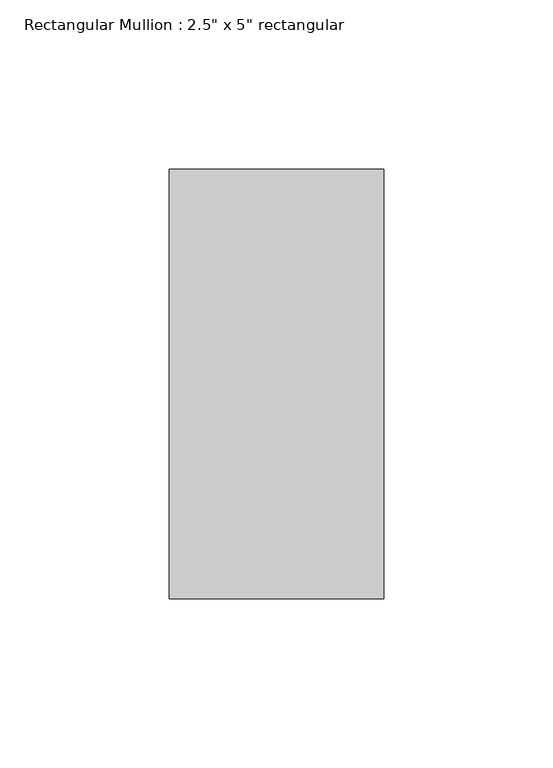
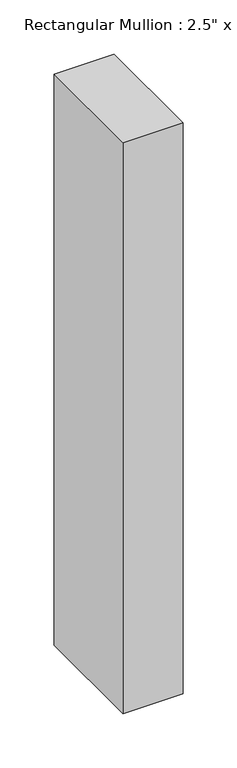
"""IFC4 building model written with IfcOpenShell, lengths in millimetres: member geometry."""

from ifc_helpers import new_model, si_unit, frame, origin, place, context, project, spatial, polyline, outline, extrude, source, transform, mapped, element, save


def member_dad99500(model_context):
    return source(origin(), model_context, "Body", "SweptSolid", [
        extrude(outline(polyline([(0.0, 63.5), (0.0, -63.5), (-63.5, -63.5), (-63.5, 63.5), (0.0, 63.5)])), frame((0.0, 0.0, -641.35), z_axis=(0.0, 0.0, 1.0), x_axis=(1.0, 0.0, 0.0)), (0.0, 0.0, 1.0), 641.35),
    ])


if __name__ == "__main__":
    model = new_model("IFC4")
    model_context = context("Model", 3, world=origin())
    ifc_project = project(units=[si_unit("LENGTHUNIT", "METRE", prefix="MILLI")], contexts=[model_context])
    site = spatial("IfcSite", under=ifc_project)
    building = spatial("IfcBuilding", under=site)
    placement = place(None, origin())
    member_shape = member_dad99500(model_context)
    element("IfcMember", 1, ObjectType="Rectangular Mullion : 2.5\" x 5\" rectangular", at=placement, inside=building, context=model_context, shape_type="MappedRepresentation", body=[
        mapped(member_shape, transform((0.0, 0.0, 0.0), x_axis=(1.0, 0.0, 0.0), y_axis=(0.0, 1.0, 0.0), z_axis=(0.0, 0.0, 1.0))),
    ])
    save(model, "model.ifc")

# Revit data of these elements
# Type "Rectangular Mullion : 2.5\" x 5\" rectangular"
#   built-in parameter 1007304 = 0.416667 (stored number, unit not read)
#   built-in parameter 1007301 = 0.104167 (stored number, unit not read)
#   built-in parameter 1007300 = 0.104167 (stored number, unit not read)
# Element 1 (IfcMember, "Rectangular Mullion : 2.5\" x 5\" rectangular")
#   Materials on its faces: "Aluminum"
# Materials
#   "Aluminum": class "Metal", colour RGB 247 247 247, transparency 0, Description = "Aluminum 6061", Cost = 0
